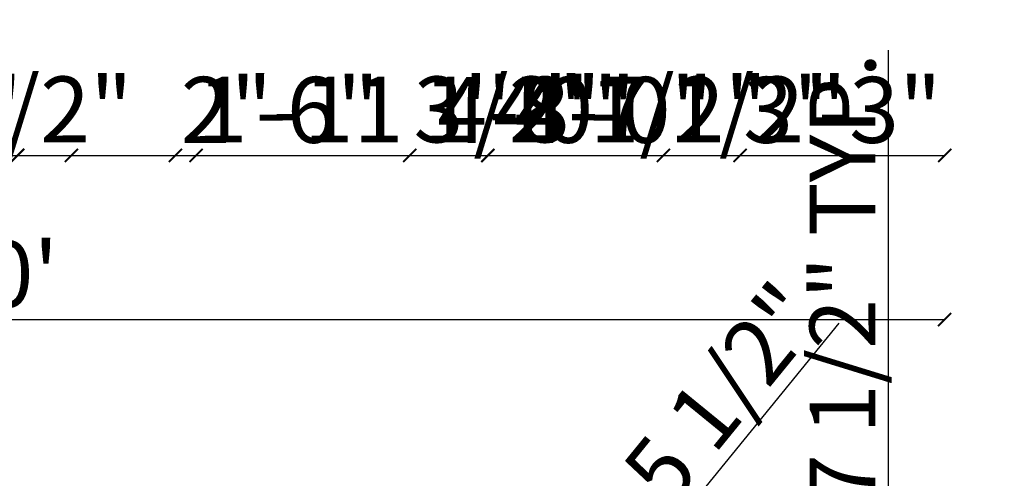
# Model space of a CAD drawing. Units: inches. Extents: x 1858 to 2399, y 1317 to 1943.
# Tile 7 of 8: x 2098 to 2285, y 1856 to 1943. Entities that reach past the tile are written whole.
import ezdxf

# ---------------------------------------------------------------- set-up
doc = ezdxf.new("R2010")
doc.units = ezdxf.units.IN
doc.layers.add('A-ANNO-DIMS', color=2, linetype='Continuous', lineweight=18)
doc.styles.get("Standard").update_dxf_attribs({"font": 'arial.ttf'})
doc.dimstyles.new('ISO-25', dxfattribs={"dimtxt": 12.5, "dimasz": 2.5, "dimexe": 1.25, "dimexo": 0.625, "dimtad": 1, "dimdec": 0, "dimlunit": 4, "dimtxsty": 'Standard', "dimblk": 'ARCHTICK', "dimcen": 2.5, "dimse1": 1, "dimse2": 1, "dimclrd": 3, "dimclrt": 4, "dimadec": 0, "dimazin": 0, "dimtfac": 1, "dimtdec": 0, "dimtmove": 0, "dimatfit": 3, "dimfxl": 1, "dimarcsym": 0})

# ---------------------------------------------------------------- blocks, each defined once
blk = doc.blocks.new('_ArchTick')
at = {"color": 0, "linetype": 'ByBlock', "const_width": 0.15}
blk.add_lwpolyline([(-0.5, -0.5), (0.5, 0.5)], dxfattribs=at)
blk = doc.blocks.new('*D14')
at = {"layer": 'A-ANNO-DIMS', "color": 0, "lineweight": -2, "transparency": 16777216}
blk.add_line((1913.38, 1886.42), (2273.38, 1886.42), dxfattribs=at)
at = {"layer": 'Defpoints', "color": 0, "transparency": 16777216}
for p in [(2273.38, 1886.42), (1913.38, 1826.41), (2273.38, 1827.14)]:
    blk.add_point(p, dxfattribs=at)
at = {"layer": 'A-ANNO-DIMS', "color": 0, "lineweight": -2, "transparency": 16777216, "xscale": 2.5, "yscale": 2.5, "zscale": 2.5, "rotation": 180}
blk.add_blockref('_ArchTick', (1913.38, 1886.42), dxfattribs=at)
at = {"layer": 'A-ANNO-DIMS', "color": 0, "lineweight": -2, "transparency": 16777216, "xscale": 2.5, "yscale": 2.5, "zscale": 2.5}
blk.add_blockref('_ArchTick', (2273.38, 1886.42), dxfattribs=at)
at = {"layer": 'A-ANNO-DIMS', "color": 0, "transparency": 16777216, "insert": (2093.38, 1893.43), "char_height": 12.5, "attachment_point": 5}
blk.add_mtext("30'", dxfattribs=at)
blk = doc.blocks.new('*D16')
at = {"layer": 'A-ANNO-DIMS', "color": 3, "lineweight": -2, "transparency": 16777216}
for p, q in [((2262.71, 1828.34), (2262.71, 1937.48)), ((2262.71, 1748.8), (2262.71, 1828.34))]:
    blk.add_line(p, q, dxfattribs=at)
at = {"layer": 'Defpoints', "color": 0, "transparency": 16777216}
for p in [(2249.76, 1828.34), (2262.71, 1828.34), (2249.76, 1748.8)]:
    blk.add_point(p, dxfattribs=at)
at = {"layer": 'A-ANNO-DIMS', "color": 3, "lineweight": -2, "transparency": 16777216, "xscale": 2.5, "yscale": 2.5, "zscale": 2.5}
for p, rotation in [((2262.71, 1828.34), 90), ((2262.71, 1748.8), 270)]:
    blk.add_blockref('_ArchTick', p, dxfattribs=dict(at, rotation=rotation))
at = {"layer": 'A-ANNO-DIMS', "color": 4, "transparency": 16777216, "insert": (2255.62, 1884.16), "char_height": 12.5, "attachment_point": 5, "rotation": 90}
blk.add_mtext('6\'-7 1/2" TYP.', dxfattribs=at)
blk = doc.blocks.new('*D33')
at = {"layer": 'A-ANNO-DIMS', "color": 3, "lineweight": -2, "transparency": 16777216}
for p, q in [((1989.86, 1917.54), (2051.43, 1917.54)), ((2051.43, 1917.54), (2117.53, 1917.54))]:
    blk.add_line(p, q, dxfattribs=at)
at = {"layer": 'Defpoints', "color": 0, "transparency": 16777216}
for p in [(2051.43, 1917.54), (1989.86, 1837.34), (2051.43, 1837.34)]:
    blk.add_point(p, dxfattribs=at)
at = {"layer": 'A-ANNO-DIMS', "color": 3, "lineweight": -2, "transparency": 16777216, "xscale": 2.5, "yscale": 2.5, "zscale": 2.5, "rotation": 180}
blk.add_blockref('_ArchTick', (1989.86, 1917.54), dxfattribs=at)
at = {"layer": 'A-ANNO-DIMS', "color": 3, "lineweight": -2, "transparency": 16777216, "xscale": 2.5, "yscale": 2.5, "zscale": 2.5}
blk.add_blockref('_ArchTick', (2051.43, 1917.54), dxfattribs=at)
at = {"layer": 'A-ANNO-DIMS', "color": 4, "transparency": 16777216, "insert": (2085.73, 1924.63), "char_height": 12.5, "attachment_point": 5}
blk.add_mtext('5\'-1 1/2"', dxfattribs=at)
blk = doc.blocks.new('*D34')
at = {"layer": 'A-ANNO-DIMS', "color": 3, "lineweight": -2, "transparency": 16777216}
blk.add_line((2051.43, 1917.54), (2107.67, 1917.54), dxfattribs=at)
at = {"layer": 'Defpoints', "color": 0, "transparency": 16777216}
for p in [(2107.67, 1917.54), (2051.43, 1837.34), (2107.67, 1837.34)]:
    blk.add_point(p, dxfattribs=at)
at = {"layer": 'A-ANNO-DIMS', "color": 3, "lineweight": -2, "transparency": 16777216, "xscale": 2.5, "yscale": 2.5, "zscale": 2.5, "rotation": 180}
blk.add_blockref('_ArchTick', (2051.43, 1917.54), dxfattribs=at)
at = {"layer": 'A-ANNO-DIMS', "color": 3, "lineweight": -2, "transparency": 16777216, "xscale": 2.5, "yscale": 2.5, "zscale": 2.5}
blk.add_blockref('_ArchTick', (2107.67, 1917.54), dxfattribs=at)
at = {"layer": 'A-ANNO-DIMS', "color": 4, "transparency": 16777216, "insert": (2079.55, 1924.55), "char_height": 12.5, "attachment_point": 5}
blk.add_mtext('4\'-8"', dxfattribs=at)
blk = doc.blocks.new('*D35')
at = {"layer": 'A-ANNO-DIMS', "color": 3, "lineweight": -2, "transparency": 16777216}
for p, q in [((2107.67, 1917.54), (2131.33, 1917.54)), ((2131.33, 1917.54), (2205.97, 1917.54))]:
    blk.add_line(p, q, dxfattribs=at)
at = {"layer": 'Defpoints', "color": 0, "transparency": 16777216}
for p in [(2131.33, 1917.54), (2107.67, 1837.34), (2131.33, 1837.34)]:
    blk.add_point(p, dxfattribs=at)
at = {"layer": 'A-ANNO-DIMS', "color": 3, "lineweight": -2, "transparency": 16777216, "xscale": 2.5, "yscale": 2.5, "zscale": 2.5, "rotation": 180}
blk.add_blockref('_ArchTick', (2107.67, 1917.54), dxfattribs=at)
at = {"layer": 'A-ANNO-DIMS', "color": 3, "lineweight": -2, "transparency": 16777216, "xscale": 2.5, "yscale": 2.5, "zscale": 2.5}
blk.add_blockref('_ArchTick', (2131.33, 1917.54), dxfattribs=at)
at = {"layer": 'A-ANNO-DIMS', "color": 4, "transparency": 16777216, "insert": (2169.9, 1924.63), "char_height": 12.5, "attachment_point": 5}
blk.add_mtext('1\'-11 1/2"', dxfattribs=at)
blk = doc.blocks.new('*D36')
at = {"layer": 'A-ANNO-DIMS', "color": 3, "lineweight": -2, "transparency": 16777216}
for p, q in [((2131.33, 1917.54), (2186.7, 1917.54)), ((2186.7, 1917.54), (2253.31, 1917.54))]:
    blk.add_line(p, q, dxfattribs=at)
at = {"layer": 'Defpoints', "color": 0, "transparency": 16777216}
for p in [(2186.7, 1917.54), (2131.33, 1837.34), (2186.7, 1837.34)]:
    blk.add_point(p, dxfattribs=at)
at = {"layer": 'A-ANNO-DIMS', "color": 3, "lineweight": -2, "transparency": 16777216, "xscale": 2.5, "yscale": 2.5, "zscale": 2.5, "rotation": 180}
blk.add_blockref('_ArchTick', (2131.33, 1917.54), dxfattribs=at)
at = {"layer": 'A-ANNO-DIMS', "color": 3, "lineweight": -2, "transparency": 16777216, "xscale": 2.5, "yscale": 2.5, "zscale": 2.5}
blk.add_blockref('_ArchTick', (2186.7, 1917.54), dxfattribs=at)
at = {"layer": 'A-ANNO-DIMS', "color": 4, "transparency": 16777216, "insert": (2221.25, 1924.63), "char_height": 12.5, "attachment_point": 5}
blk.add_mtext('4\'-7 1/2"', dxfattribs=at)
blk = doc.blocks.new('*D37')
at = {"layer": 'A-ANNO-DIMS', "color": 3, "lineweight": -2, "transparency": 16777216}
blk.add_line((2186.7, 1917.54), (2234.56, 1917.54), dxfattribs=at)
at = {"layer": 'Defpoints', "color": 0, "transparency": 16777216}
for p in [(2234.56, 1917.54), (2186.7, 1837.34), (2234.56, 1837.34)]:
    blk.add_point(p, dxfattribs=at)
at = {"layer": 'A-ANNO-DIMS', "color": 3, "lineweight": -2, "transparency": 16777216, "xscale": 2.5, "yscale": 2.5, "zscale": 2.5, "rotation": 180}
blk.add_blockref('_ArchTick', (2186.7, 1917.54), dxfattribs=at)
at = {"layer": 'A-ANNO-DIMS', "color": 3, "lineweight": -2, "transparency": 16777216, "xscale": 2.5, "yscale": 2.5, "zscale": 2.5}
blk.add_blockref('_ArchTick', (2234.56, 1917.54), dxfattribs=at)
at = {"layer": 'A-ANNO-DIMS', "color": 4, "transparency": 16777216, "insert": (2210.63, 1924.55), "char_height": 12.5, "attachment_point": 5}
blk.add_mtext('4\'-0"', dxfattribs=at)
blk = doc.blocks.new('*D38')
at = {"layer": 'A-ANNO-DIMS', "color": 3, "lineweight": -2, "transparency": 16777216}
blk.add_line((2234.56, 1917.54), (2273.38, 1917.54), dxfattribs=at)
at = {"layer": 'Defpoints', "color": 0, "transparency": 16777216}
for p in [(2273.38, 1917.54), (2234.56, 1837.34), (2273.38, 1837.34)]:
    blk.add_point(p, dxfattribs=at)
at = {"layer": 'A-ANNO-DIMS', "color": 3, "lineweight": -2, "transparency": 16777216, "xscale": 2.5, "yscale": 2.5, "zscale": 2.5, "rotation": 180}
blk.add_blockref('_ArchTick', (2234.56, 1917.54), dxfattribs=at)
at = {"layer": 'A-ANNO-DIMS', "color": 3, "lineweight": -2, "transparency": 16777216, "xscale": 2.5, "yscale": 2.5, "zscale": 2.5}
blk.add_blockref('_ArchTick', (2273.38, 1917.54), dxfattribs=at)
at = {"layer": 'A-ANNO-DIMS', "color": 4, "transparency": 16777216, "insert": (2253.97, 1924.55), "char_height": 12.5, "attachment_point": 5}
blk.add_mtext('3\'-3"', dxfattribs=at)
blk = doc.blocks.new('*D50')
at = {"layer": 'A-ANNO-DIMS', "color": 3, "lineweight": -2, "transparency": 16777216}
for p, q in [((2097.46, 1917.54), (2127.41, 1917.54)), ((2127.41, 1917.54), (2164.6, 1917.54))]:
    blk.add_line(p, q, dxfattribs=at)
at = {"layer": 'Defpoints', "color": 0, "transparency": 16777216}
for p in [(2127.41, 1917.54), (2097.46, 1563.34), (2127.41, 1563.34)]:
    blk.add_point(p, dxfattribs=at)
at = {"layer": 'A-ANNO-DIMS', "color": 3, "lineweight": -2, "transparency": 16777216, "xscale": 2.5, "yscale": 2.5, "zscale": 2.5, "rotation": 180}
blk.add_blockref('_ArchTick', (2097.46, 1917.54), dxfattribs=at)
at = {"layer": 'A-ANNO-DIMS', "color": 3, "lineweight": -2, "transparency": 16777216, "xscale": 2.5, "yscale": 2.5, "zscale": 2.5}
blk.add_blockref('_ArchTick', (2127.41, 1917.54), dxfattribs=at)
at = {"layer": 'A-ANNO-DIMS', "color": 4, "transparency": 16777216, "insert": (2147.25, 1924.55), "char_height": 12.5, "attachment_point": 5}
blk.add_mtext('2\'-6"', dxfattribs=at)
blk = doc.blocks.new('*D51')
at = {"layer": 'A-ANNO-DIMS', "color": 3, "lineweight": -2, "transparency": 16777216}
for p, q in [((2127.41, 1917.54), (2171.86, 1917.54)), ((2171.86, 1917.54), (2237.95, 1917.54))]:
    blk.add_line(p, q, dxfattribs=at)
at = {"layer": 'Defpoints', "color": 0, "transparency": 16777216}
for p in [(2171.86, 1917.54), (2127.41, 1563.34), (2171.86, 1563.34)]:
    blk.add_point(p, dxfattribs=at)
at = {"layer": 'A-ANNO-DIMS', "color": 3, "lineweight": -2, "transparency": 16777216, "xscale": 2.5, "yscale": 2.5, "zscale": 2.5, "rotation": 180}
blk.add_blockref('_ArchTick', (2127.41, 1917.54), dxfattribs=at)
at = {"layer": 'A-ANNO-DIMS', "color": 3, "lineweight": -2, "transparency": 16777216, "xscale": 2.5, "yscale": 2.5, "zscale": 2.5}
blk.add_blockref('_ArchTick', (2171.86, 1917.54), dxfattribs=at)
at = {"layer": 'A-ANNO-DIMS', "color": 4, "transparency": 16777216, "insert": (2206.15, 1924.63), "char_height": 12.5, "attachment_point": 5}
blk.add_mtext('3\'-8 1/2"', dxfattribs=at)
blk = doc.blocks.new('*D52')
at = {"layer": 'A-ANNO-DIMS', "color": 3, "lineweight": -2, "transparency": 16777216}
blk.add_line((2171.86, 1917.54), (2220, 1917.54), dxfattribs=at)
at = {"layer": 'Defpoints', "color": 0, "transparency": 16777216}
for p in [(2220, 1917.54), (2171.86, 1563.34), (2220, 1563.34)]:
    blk.add_point(p, dxfattribs=at)
at = {"layer": 'A-ANNO-DIMS', "color": 3, "lineweight": -2, "transparency": 16777216, "xscale": 2.5, "yscale": 2.5, "zscale": 2.5, "rotation": 180}
blk.add_blockref('_ArchTick', (2171.86, 1917.54), dxfattribs=at)
at = {"layer": 'A-ANNO-DIMS', "color": 3, "lineweight": -2, "transparency": 16777216, "xscale": 2.5, "yscale": 2.5, "zscale": 2.5}
blk.add_blockref('_ArchTick', (2220, 1917.54), dxfattribs=at)
at = {"layer": 'A-ANNO-DIMS', "color": 4, "transparency": 16777216, "insert": (2195.93, 1924.55), "char_height": 12.5, "attachment_point": 5}
blk.add_mtext('4\'-0"', dxfattribs=at)
blk = doc.blocks.new('*D60')
at = {"layer": 'A-ANNO-DIMS', "color": 3, "lineweight": -2, "transparency": 16777216}
for p in [(2253.32, 1885.76), (2181.85, 1798.12)]:
    blk.add_line(p, (2185.3, 1802.34), dxfattribs=at)
at = {"layer": 'Defpoints', "color": 0, "transparency": 16777216}
for p in [(2185.3, 1802.34), (2181.85, 1798.12)]:
    blk.add_point(p, dxfattribs=at)
at = {"layer": 'A-ANNO-DIMS', "color": 3, "lineweight": -2, "transparency": 16777216, "xscale": 2.5, "yscale": 2.5, "zscale": 2.5, "rotation": 230.8077101952448}
blk.add_blockref('_ArchTick', (2185.3, 1802.34), dxfattribs=at)
at = {"layer": 'A-ANNO-DIMS', "color": 4, "transparency": 16777216, "insert": (2215.4, 1850.47), "char_height": 12.5, "attachment_point": 5, "rotation": 50.8077}
blk.add_mtext('2X R0\'-5 1/2"', dxfattribs=at)

msp = doc.modelspace()

# ---------------------------------------------------------------- dimensions: what is measured, and where the dimension line sits
at = {"layer": 'A-ANNO-DIMS'}
for base, p1, p2, override, picture, middle in [((2051.43, 1917.54), (1989.86, 1837.34), (2051.43, 1837.34), {"dimdec": 1, "dimlfac": 1, "dimrnd": 0, "dimzin": 1, "dimdsep": 46, "dimlunit": 4, "dimfrac": 2}, '*D33', (2085.73, 1924.63)), ((2131.33, 1917.54), (2107.67, 1837.34), (2131.33, 1837.34), {"dimdec": 1, "dimlfac": 1, "dimrnd": 0, "dimzin": 1, "dimdsep": 46, "dimlunit": 4, "dimfrac": 2}, '*D35', (2169.9, 1924.63)), ((2171.8564, 1917.5395), (2127.4089, 1563.3395), (2171.8564, 1563.3395), {"dimdec": 1, "dimlfac": 1, "dimrnd": 0, "dimzin": 1, "dimdsep": 46, "dimlunit": 4, "dimfrac": 2}, '*D51', (2206.1547, 1924.6319)), ((2186.7, 1917.54), (2131.33, 1837.34), (2186.7, 1837.34), {"dimdec": 1, "dimlfac": 1, "dimrnd": 0, "dimzin": 1, "dimdsep": 46, "dimlunit": 4, "dimfrac": 2}, '*D36', (2221.25, 1924.63)), ((2107.67, 1917.54), (2051.43, 1837.34), (2107.67, 1837.34), {"dimdec": 1, "dimlfac": 1, "dimrnd": 0, "dimzin": 1, "dimdsep": 46, "dimlunit": 4, "dimfrac": 2}, '*D34', (2079.55, 1924.55)), ((2127.4089, 1917.5395), (2097.4626, 1563.3395), (2127.4089, 1563.3395), {"dimdec": 1, "dimlfac": 1, "dimrnd": 0, "dimzin": 1, "dimdsep": 46, "dimlunit": 4, "dimfrac": 2}, '*D50', (2147.2545, 1924.5467)), ((2220, 1917.54), (2171.86, 1563.34), (2220, 1563.34), {"dimdec": 1, "dimlfac": 1, "dimrnd": 0, "dimzin": 1, "dimdsep": 46, "dimlunit": 4, "dimfrac": 2}, '*D52', (2195.93, 1924.55)), ((2234.56, 1917.54), (2186.7, 1837.34), (2234.56, 1837.34), {"dimdec": 1, "dimlfac": 1, "dimrnd": 0, "dimzin": 1, "dimdsep": 46, "dimlunit": 4, "dimfrac": 2}, '*D37', (2210.63, 1924.55)), ((2273.38, 1917.54), (2234.56, 1837.34), (2273.38, 1837.34), {"dimdec": 1, "dimlfac": 1, "dimrnd": 0, "dimzin": 1, "dimdsep": 46, "dimlunit": 4, "dimfrac": 2}, '*D38', (2253.97, 1924.55)), ((2273.38, 1886.42), (1913.38, 1826.41), (2273.38, 1827.14), {"dimclrd": 0, "dimclre": 0, "dimclrt": 0}, '*D14', (2093.38, 1893.43))]:
    dim = msp.add_linear_dim(base=base, p1=p1, p2=p2, dimstyle='ISO-25', override=override, dxfattribs=at)
    dim.commit()
    dim.dimension.update_dxf_attribs({"geometry": picture, "text_midpoint": middle})
dim = msp.add_linear_dim(base=(2262.71, 1828.34), p1=(2249.76, 1748.8), p2=(2249.76, 1828.34), angle=90, text='<> TYP.', dimstyle='ISO-25', override={"dimdec": 1, "dimlfac": 1, "dimrnd": 0, "dimzin": 1, "dimdsep": 46, "dimlunit": 4, "dimfrac": 2}, dxfattribs=at)
dim.commit()
dim.dimension.update_dxf_attribs({"geometry": '*D16', "text_midpoint": (2255.62, 1884.16)})
dim = msp.add_radius_dim(center=(2181.85, 1798.12), mpoint=(2185.3, 1802.34), text='2X <>', dimstyle='ISO-25', override={"dimdec": 1, "dimlfac": 1, "dimrnd": 0, "dimzin": 1, "dimdsep": 46, "dimlunit": 4, "dimfrac": 2}, dxfattribs=at)
dim.commit()
dim.dimension.update_dxf_attribs({"geometry": '*D60', "text_midpoint": (2215.4, 1850.47)})

doc.saveas('drawing.dxf')
